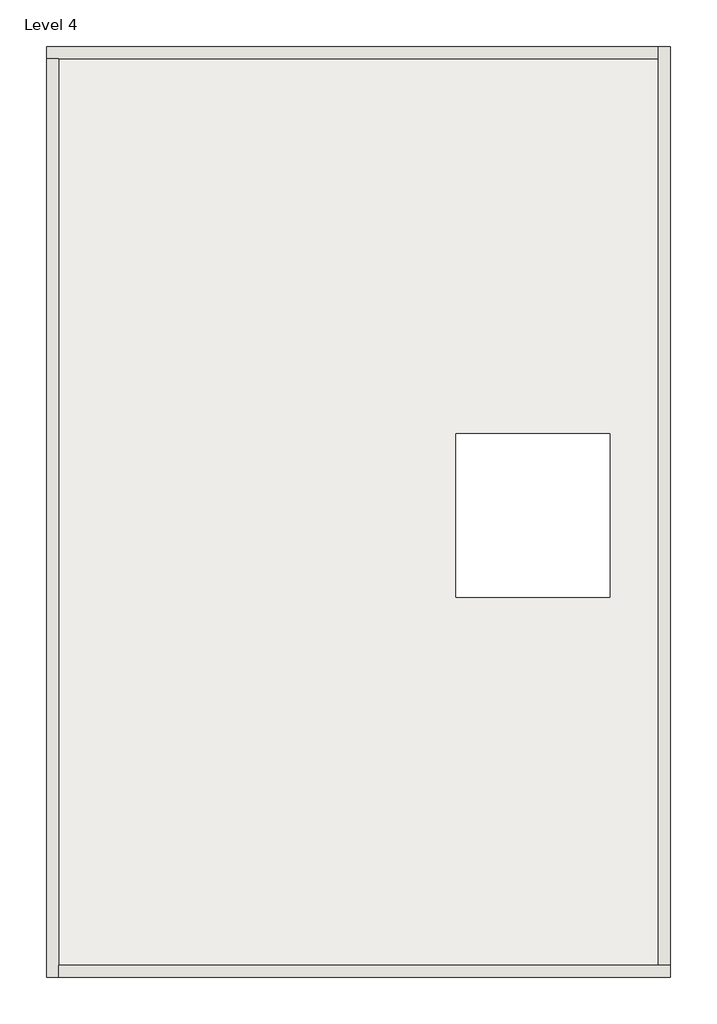
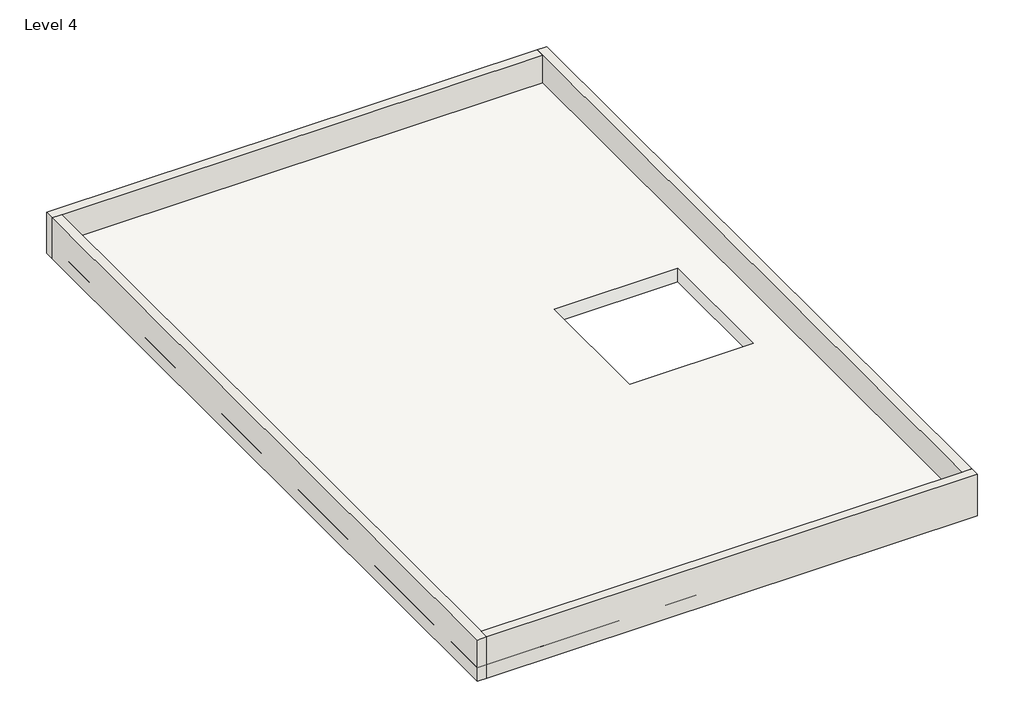
# One storey, incomplete: 4 walls, 1 roof.
"""IFC4 building model written with IfcOpenShell, lengths in millimetres."""

from ifc_helpers import new_model, si_unit, frame, origin, place, context, project, spatial, polyline, outline, extrude, faceted_brep, element, save

model = new_model("IFC4")

# Units and contexts
model_context = context("Model", 3, world=origin())
ifc_project = project(units=[si_unit("LENGTHUNIT", "METRE", prefix="MILLI")], contexts=[model_context])

# Site, building, storey
site = spatial("IfcSite", under=ifc_project)
building = spatial("IfcBuilding", under=site)
storey = spatial("IfcBuildingStorey", under=building, Name="Level 4", Elevation=9144.0)

# Roof
placement = place(None, origin())
element("IfcRoof", 1, ObjectType="Generic - 12\"", at=placement, inside=storey, context=model_context, shape_type="SweptSolid", body=[
    extrude(outline(polyline([(-3416.9711241, 17066.5344295), (-3416.9711241, 1420.1344295), (-13907.1711241, 1420.1344295), (-13907.1711241, 17066.5344295), (-3416.9711241, 17066.5344295)]), holes=[polyline([(-4429.4532065, 10554.8963064), (-7020.2532065, 10554.8963064), (-7020.2532065, 7811.6963064), (-4429.4532065, 7811.6963064), (-4429.4532065, 10554.8963064)])]), frame((0.0, 0.0, 9144.0), z_axis=(0.0, 0.0, 1.0), x_axis=(1.0, 0.0, 0.0)), (0.0, 0.0, 1.0), 304.8),
])

# Walls
element("IfcWall", 2, ObjectType="Generic -4.5\" p", at=placement, inside=storey, context=model_context, shape_type="Brep", body=[
    faceted_brep([(-13907.1711241, 16863.3344295, 9144.0), (-13703.9711241, 16863.3344295, 9144.0), (-3620.1711241, 16863.3344295, 9144.0), (-3620.1711241, 16863.3344295, 10058.4), (-13703.9711241, 16863.3344295, 10058.4), (-13907.1711241, 16863.3344295, 10058.4), (-13907.1711241, 17066.5344295, 9144.0), (-13907.1711241, 17066.5344295, 10058.4), (-3620.1711241, 17066.5344295, 10058.4), (-3620.1711241, 17066.5344295, 9144.0)], [[[0, 1, 2, 3, 4, 5]], [[6, 7, 8, 9]], [[2, 1, 0, 6, 9]], [[5, 4, 3, 8, 7]], [[0, 5, 7, 6]], [[3, 2, 9, 8]]]),
])
element("IfcWall", 3, ObjectType="Generic -4.5\" p", at=placement, inside=storey, context=model_context, shape_type="Brep", body=[
    faceted_brep([(-13703.9711241, 1420.1344295, 9144.0), (-13703.9711241, 1623.3344295, 9144.0), (-13703.9711241, 16863.3344295, 9144.0), (-13703.9711241, 16863.3344295, 10058.4), (-13703.9711241, 1623.3344295, 10058.4), (-13703.9711241, 1420.1344295, 10058.4), (-13907.1711241, 1420.1344295, 9144.0), (-13907.1711241, 1420.1344295, 10058.4), (-13907.1711241, 16863.3344295, 10058.4), (-13907.1711241, 16863.3344295, 9144.0)], [[[0, 1, 2, 3, 4, 5]], [[6, 7, 8, 9]], [[2, 1, 0, 6, 9]], [[5, 4, 3, 8, 7]], [[0, 5, 7, 6]], [[3, 2, 9, 8]]]),
])
element("IfcWall", 4, ObjectType="Generic -4.5\" p", at=placement, inside=storey, context=model_context, shape_type="Brep", body=[
    faceted_brep([(-3416.9711241, 1623.3344295, 9144.0), (-3620.1711241, 1623.3344295, 9144.0), (-13703.9711241, 1623.3344295, 9144.0), (-13703.9711241, 1623.3344295, 10058.4), (-3620.1711241, 1623.3344295, 10058.4), (-3416.9711241, 1623.3344295, 10058.4), (-3416.9711241, 1420.1344295, 9144.0), (-3416.9711241, 1420.1344295, 10058.4), (-13703.9711241, 1420.1344295, 10058.4), (-13703.9711241, 1420.1344295, 9144.0)], [[[0, 1, 2, 3, 4, 5]], [[6, 7, 8, 9]], [[2, 1, 0, 6, 9]], [[5, 4, 3, 8, 7]], [[0, 5, 7, 6]], [[3, 2, 9, 8]]]),
])
element("IfcWall", 5, ObjectType="Generic -4.5\" p", at=placement, inside=storey, context=model_context, shape_type="Brep", body=[
    faceted_brep([(-3620.1711241, 17066.5344295, 9144.0), (-3620.1711241, 16863.3344295, 9144.0), (-3620.1711241, 1623.3344295, 9144.0), (-3620.1711241, 1623.3344295, 10058.4), (-3620.1711241, 16863.3344295, 10058.4), (-3620.1711241, 17066.5344295, 10058.4), (-3416.9711241, 17066.5344295, 9144.0), (-3416.9711241, 17066.5344295, 10058.4), (-3416.9711241, 1623.3344295, 10058.4), (-3416.9711241, 1623.3344295, 9144.0)], [[[0, 1, 2, 3, 4, 5]], [[6, 7, 8, 9]], [[2, 1, 0, 6, 9]], [[5, 4, 3, 8, 7]], [[0, 5, 7, 6]], [[3, 2, 9, 8]]]),
])

save(model, "model.ifc")

# Revit data of these elements
# Type "Generic - 12\""
#   Assembly Code = "B1020"
#   Layers, outside or top first: 1' - 0" no material (function 1)
# Type "Generic -4.5\" p"
#   Assembly Code = "B2010"
#   Layers, outside or top first: 0' - 8" no material (function 1)
# Element 1 (IfcRoof, "Generic - 12\"")
#   built-in parameter 1001705 = 31 (stored number, unit not read)
#   built-in parameter 1001710 = 33615
#   Phase Created = New Construction
#   Materials on its faces: "Default Roof"
# Elements 2, 3, 4, 5 (IfcWall, "Generic -4.5\" p")
#   Top Offset = 0' - 0"
#   Base Offset = 0' - 0"
#   Unconnected Height = 3' - 0"
#   wall height = 3' - 0"
#   Phase Created = New Construction
#   Base Constraint = Level 4
#   Materials on its faces: "Default Wall", "Earth"
# Materials
#   "Default Roof": colour RGB 88 101 114, transparency 0, Cost = 0
#   "Default Wall": colour RGB 128 128 128, transparency 0, Cost = 0
#   "Earth": class "Generic", colour RGB 97 75 62, transparency 0, Description = "Soil", Cost = 0
